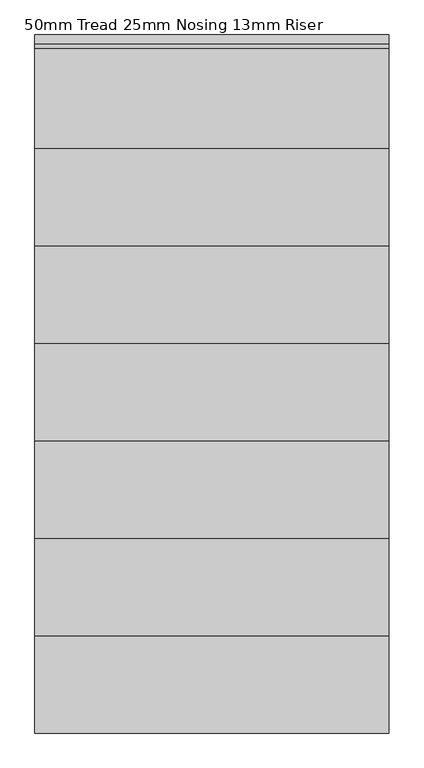
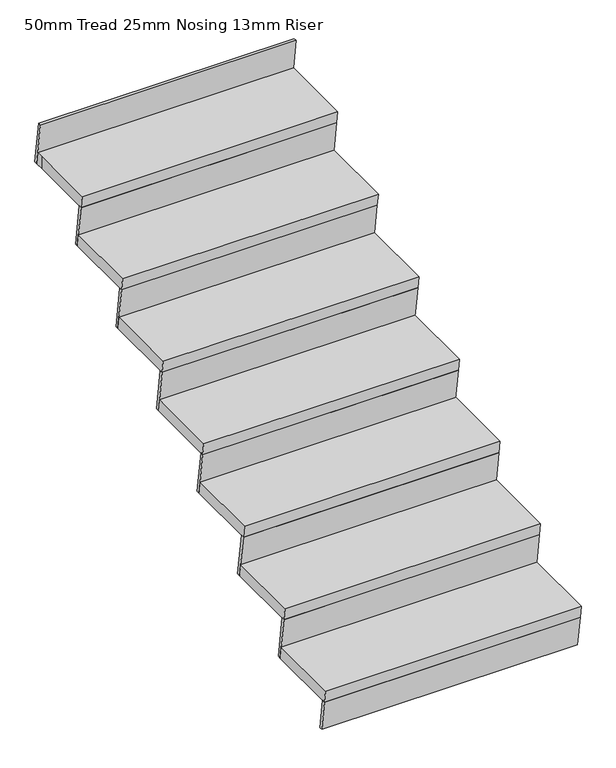
"""IFC4 building model written with IfcOpenShell, lengths in millimetres: stair flight geometry, 50mm Tread 25mm Nosing 13mm Riser."""

from ifc_helpers import new_model, si_unit, origin, place, context, project, spatial, faceted_brep, source, transform, mapped, element, save


def stair_flight_50mm_tread_25mm_nosing_13mm_riser_88d6afc4(model_context):
    return source(origin(), model_context, "Body", "Brep", [
        faceted_brep([(-3562.8939506, 9198.7482221, 173.9130435), (-3562.8939506, 9205.9357221, 123.9130435), (-4562.9197318, 9205.9357221, 123.9130435), (-4562.9197318, 9198.7482221, 173.9130435), (-4562.9197318, 8898.7482221, 173.9130435), (-3562.8939506, 8898.7482221, 173.9130435), (-3562.8939506, 8905.9357221, 123.9130435), (-4562.9197318, 8905.9357221, 123.9130435)], [[[0, 1, 2, 3]], [[3, 4, 5, 0]], [[2, 1, 6, 7]], [[4, 3, 2, 7]], [[0, 5, 6, 1]], [[5, 4, 7, 6]]]),
        faceted_brep([(-3562.8939506, 8905.9357221, 123.9130435), (-3562.8939506, 8923.7482221, 0.0), (-3562.8939506, 8936.3767121, 0.0), (-3562.8939506, 8918.5642121, 123.9130435), (-4562.9197318, 8905.9357221, 123.9130435), (-4562.9197318, 8918.5642121, 123.9130435), (-4562.9197318, 8936.3767121, 0.0), (-4562.9197318, 8923.7482221, 0.0)], [[[0, 1, 2, 3]], [[4, 5, 6, 7]], [[1, 0, 4, 7]], [[2, 1, 7, 6]], [[3, 2, 6, 5]], [[0, 3, 5, 4]]]),
        faceted_brep([(-3562.8939506, 9180.9357221, 297.826087), (-3562.8939506, 9205.9357221, 123.9130435), (-3562.8939506, 9218.5642121, 123.9130435), (-3562.8939506, 9193.5642121, 297.826087), (-4562.9197318, 9180.9357221, 297.826087), (-4562.9197318, 9193.5642121, 297.826087), (-4562.9197318, 9218.5642121, 123.9130435), (-4562.9197318, 9205.9357221, 123.9130435)], [[[0, 1, 2, 3]], [[4, 5, 6, 7]], [[1, 0, 4, 7]], [[2, 1, 7, 6]], [[3, 2, 6, 5]], [[0, 3, 5, 4]]]),
        faceted_brep([(-4562.9197318, 9473.7482221, 347.826087), (-4562.9197318, 9173.7482221, 347.826087), (-3562.8939506, 9173.7482221, 347.826087), (-3562.8939506, 9473.7482221, 347.826087), (-4562.9197318, 9480.9357221, 297.826087), (-3562.8939506, 9480.9357221, 297.826087), (-3562.8939506, 9180.9357221, 297.826087), (-4562.9197318, 9180.9357221, 297.826087)], [[[0, 1, 2, 3]], [[4, 5, 6, 7]], [[1, 0, 4, 7]], [[3, 2, 6, 5]], [[3, 5, 4, 0]], [[2, 1, 7, 6]]]),
        faceted_brep([(-3562.8939506, 9455.9357221, 471.7391304), (-3562.8939506, 9480.9357221, 297.826087), (-3562.8939506, 9493.5642121, 297.826087), (-3562.8939506, 9468.5642121, 471.7391304), (-4562.9197318, 9455.9357221, 471.7391304), (-4562.9197318, 9468.5642121, 471.7391304), (-4562.9197318, 9493.5642121, 297.826087), (-4562.9197318, 9480.9357221, 297.826087)], [[[0, 1, 2, 3]], [[4, 5, 6, 7]], [[1, 0, 4, 7]], [[2, 1, 7, 6]], [[3, 2, 6, 5]], [[0, 3, 5, 4]]]),
        faceted_brep([(-4562.9197318, 9748.7482221, 521.7391304), (-4562.9197318, 9448.7482221, 521.7391304), (-3562.8939506, 9448.7482221, 521.7391304), (-3562.8939506, 9748.7482221, 521.7391304), (-4562.9197318, 9755.9357221, 471.7391304), (-3562.8939506, 9755.9357221, 471.7391304), (-3562.8939506, 9455.9357221, 471.7391304), (-4562.9197318, 9455.9357221, 471.7391304)], [[[0, 1, 2, 3]], [[4, 5, 6, 7]], [[1, 0, 4, 7]], [[3, 2, 6, 5]], [[3, 5, 4, 0]], [[2, 1, 7, 6]]]),
        faceted_brep([(-3562.8939506, 9730.9357221, 645.6521739), (-3562.8939506, 9755.9357221, 471.7391304), (-3562.8939506, 9768.5642121, 471.7391304), (-3562.8939506, 9743.5642121, 645.6521739), (-4562.9197318, 9730.9357221, 645.6521739), (-4562.9197318, 9743.5642121, 645.6521739), (-4562.9197318, 9768.5642121, 471.7391304), (-4562.9197318, 9755.9357221, 471.7391304)], [[[0, 1, 2, 3]], [[4, 5, 6, 7]], [[1, 0, 4, 7]], [[2, 1, 7, 6]], [[3, 2, 6, 5]], [[0, 3, 5, 4]]]),
        faceted_brep([(-4562.9197318, 10023.7482221, 695.6521739), (-4562.9197318, 9723.7482221, 695.6521739), (-3562.8939506, 9723.7482221, 695.6521739), (-3562.8939506, 10023.7482221, 695.6521739), (-4562.9197318, 10030.9357221, 645.6521739), (-3562.8939506, 10030.9357221, 645.6521739), (-3562.8939506, 9730.9357221, 645.6521739), (-4562.9197318, 9730.9357221, 645.6521739)], [[[0, 1, 2, 3]], [[4, 5, 6, 7]], [[1, 0, 4, 7]], [[3, 2, 6, 5]], [[3, 5, 4, 0]], [[2, 1, 7, 6]]]),
        faceted_brep([(-3562.8939506, 10005.9357221, 819.5652174), (-3562.8939506, 10030.9357221, 645.6521739), (-3562.8939506, 10043.5642121, 645.6521739), (-3562.8939506, 10018.5642121, 819.5652174), (-4562.9197318, 10005.9357221, 819.5652174), (-4562.9197318, 10018.5642121, 819.5652174), (-4562.9197318, 10043.5642121, 645.6521739), (-4562.9197318, 10030.9357221, 645.6521739)], [[[0, 1, 2, 3]], [[4, 5, 6, 7]], [[1, 0, 4, 7]], [[2, 1, 7, 6]], [[3, 2, 6, 5]], [[0, 3, 5, 4]]]),
        faceted_brep([(-4562.9197318, 10298.7482221, 869.5652174), (-4562.9197318, 9998.7482221, 869.5652174), (-3562.8939506, 9998.7482221, 869.5652174), (-3562.8939506, 10298.7482221, 869.5652174), (-4562.9197318, 10305.9357221, 819.5652174), (-3562.8939506, 10305.9357221, 819.5652174), (-3562.8939506, 10005.9357221, 819.5652174), (-4562.9197318, 10005.9357221, 819.5652174)], [[[0, 1, 2, 3]], [[4, 5, 6, 7]], [[1, 0, 4, 7]], [[3, 2, 6, 5]], [[3, 5, 4, 0]], [[2, 1, 7, 6]]]),
        faceted_brep([(-3562.8939506, 10280.9357221, 993.4782609), (-3562.8939506, 10305.9357221, 819.5652174), (-3562.8939506, 10318.5642121, 819.5652174), (-3562.8939506, 10293.5642121, 993.4782609), (-4562.9197318, 10280.9357221, 993.4782609), (-4562.9197318, 10293.5642121, 993.4782609), (-4562.9197318, 10318.5642121, 819.5652174), (-4562.9197318, 10305.9357221, 819.5652174)], [[[0, 1, 2, 3]], [[4, 5, 6, 7]], [[1, 0, 4, 7]], [[2, 1, 7, 6]], [[3, 2, 6, 5]], [[0, 3, 5, 4]]]),
        faceted_brep([(-4562.9197318, 10573.7482221, 1043.4782609), (-4562.9197318, 10273.7482221, 1043.4782609), (-3562.8939506, 10273.7482221, 1043.4782609), (-3562.8939506, 10573.7482221, 1043.4782609), (-4562.9197318, 10580.9357221, 993.4782609), (-3562.8939506, 10580.9357221, 993.4782609), (-3562.8939506, 10280.9357221, 993.4782609), (-4562.9197318, 10280.9357221, 993.4782609)], [[[0, 1, 2, 3]], [[4, 5, 6, 7]], [[1, 0, 4, 7]], [[3, 2, 6, 5]], [[3, 5, 4, 0]], [[2, 1, 7, 6]]]),
        faceted_brep([(-3562.8939506, 10830.9357221, 1341.3043478), (-3562.8939506, 10855.9357221, 1167.3913043), (-3562.8939506, 10868.5642121, 1167.3913043), (-3562.8939506, 10843.5642121, 1341.3043478), (-4562.9197318, 10830.9357221, 1341.3043478), (-4562.9197318, 10843.5642121, 1341.3043478), (-4562.9197318, 10868.5642121, 1167.3913043), (-4562.9197318, 10855.9357221, 1167.3913043)], [[[0, 1, 2, 3]], [[4, 5, 6, 7]], [[1, 0, 4, 7]], [[2, 1, 7, 6]], [[3, 2, 6, 5]], [[0, 3, 5, 4]]]),
        faceted_brep([(-3562.8939506, 10555.9357221, 1167.3913043), (-3562.8939506, 10580.9357221, 993.4782609), (-3562.8939506, 10593.5642121, 993.4782609), (-3562.8939506, 10568.5642121, 1167.3913043), (-4562.9197318, 10555.9357221, 1167.3913043), (-4562.9197318, 10568.5642121, 1167.3913043), (-4562.9197318, 10593.5642121, 993.4782609), (-4562.9197318, 10580.9357221, 993.4782609)], [[[0, 1, 2, 3]], [[4, 5, 6, 7]], [[1, 0, 4, 7]], [[2, 1, 7, 6]], [[3, 2, 6, 5]], [[0, 3, 5, 4]]]),
        faceted_brep([(-4562.9197318, 10848.7482221, 1217.3913043), (-4562.9197318, 10823.7482221, 1217.3913043), (-4562.9197318, 10548.7482221, 1217.3913043), (-3562.8939506, 10548.7482221, 1217.3913043), (-3562.8939506, 10848.7482221, 1217.3913043), (-4562.9197318, 10855.9357221, 1167.3913043), (-3562.8939506, 10855.9357221, 1167.3913043), (-3562.8939506, 10555.9357221, 1167.3913043), (-4562.9197318, 10555.9357221, 1167.3913043), (-4562.9197318, 10823.7482221, 1167.3913043)], [[[0, 1, 2, 3, 4]], [[5, 6, 7, 8, 9]], [[1, 0, 5, 9]], [[2, 1, 9, 8]], [[4, 3, 7, 6]], [[4, 6, 5, 0]], [[3, 2, 8, 7]]]),
    ])


if __name__ == "__main__":
    model = new_model("IFC4")
    model_context = context("Model", 3, world=origin())
    ifc_project = project(units=[si_unit("LENGTHUNIT", "METRE", prefix="MILLI")], contexts=[model_context])
    site = spatial("IfcSite", under=ifc_project)
    building = spatial("IfcBuilding", under=site)
    placement = place(None, origin())
    stair_flight_50mm_tread_25mm_nosing_13mm_riser_shape = stair_flight_50mm_tread_25mm_nosing_13mm_riser_88d6afc4(model_context)
    element("IfcStairFlight", 1, ObjectType="50mm Tread 25mm Nosing 13mm Riser", at=placement, inside=building, context=model_context, shape_type="MappedRepresentation", body=[
        mapped(stair_flight_50mm_tread_25mm_nosing_13mm_riser_shape, transform((0.0, 0.0, 0.0), x_axis=(1.0, 0.0, 0.0), y_axis=(0.0, 1.0, 0.0), z_axis=(0.0, 0.0, 1.0))),
    ])
    save(model, "model.ifc")
